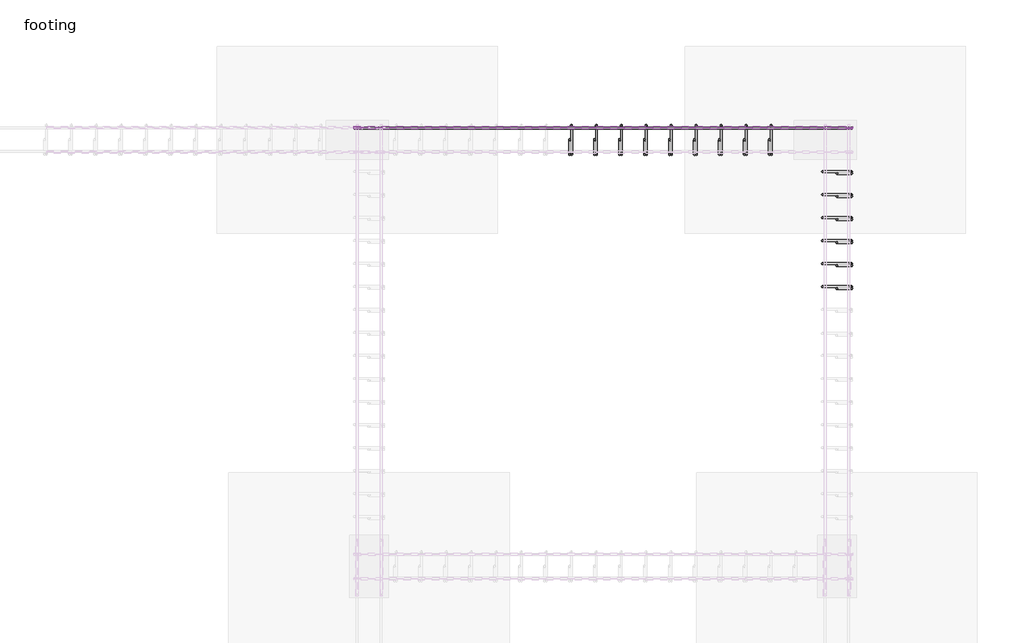
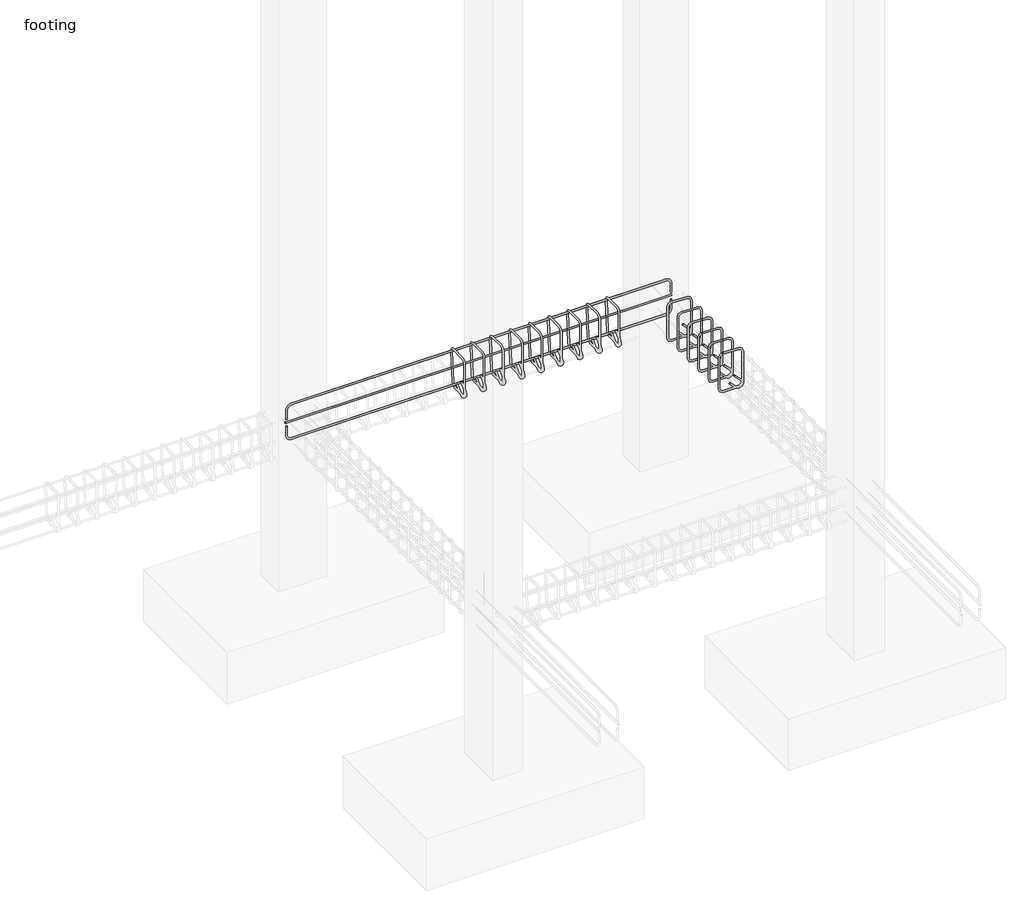
# One storey, part 21 of 21: 18 reinforcing bars.
"""IFC4 building model written with IfcOpenShell, lengths in millimetres."""

from ifc_helpers import new_model, si_unit, point, frame, origin, place, context, project, spatial, polyline, circle_curve, trimmed, segment, composite_curve, element, save
from ifc_brep_helpers import swept_disk

model = new_model("IFC4")

# Units and contexts
model_context = context("Model", 3, world=origin())
ifc_project = project(units=[si_unit("LENGTHUNIT", "METRE", prefix="MILLI")], contexts=[model_context])

# Site, building, storey
site = spatial("IfcSite", under=ifc_project)
building = spatial("IfcBuilding", under=site)
storey = spatial("IfcBuildingStorey", under=building, Name="footing", Elevation=-1524.0)

# Reinforcing bars
placement = place(None, origin())
element("IfcReinforcingBar", 1, at=placement, inside=storey, context=model_context, shape_type="SolidModel", body=[
    swept_disk(composite_curve([segment(polyline([(-4722.5521673, 11058.8872086, -236.1172592), (-4722.5521673, 11058.8872086, -312.3172592)]), True, "CONTINUOUS"), segment(trimmed(circle_curve(frame((-4767.0021673, 11058.8872086, -312.3172592), z_axis=(0.0, 1.0, -2.1166279873208456e-12), x_axis=(44.44999999999982, 0.0, 0.0)), 44.45), [point((-4722.5521673, 11058.8872086, -312.3172592))], [point((-4767.0021673, 11058.8872086, -356.7672592))], True, "CARTESIAN"), True, "CONTINUOUS"), segment(polyline([(-4767.0021673, 11058.8872086, -356.7672592), (-7917.3959173, 11058.8872086, -356.7672592)]), True, "CONTINUOUS"), segment(trimmed(circle_curve(frame((-7917.3959173, 11058.8872086, -312.3172592), z_axis=(0.0, 1.0, -2.1166279873208456e-12), x_axis=(0.0, 0.0, -44.44999999999999)), 44.45), [point((-7917.3959173, 11058.8872086, -356.7672592))], [point((-7961.8459173, 11058.8872086, -312.3172592))], True, "CARTESIAN"), True, "CONTINUOUS"), segment(polyline([(-7961.8459173, 11058.8872086, -312.3172592), (-7961.8459173, 11058.8872086, -236.1172592)]), True, "CONTINUOUS")], self_intersect=False), 6.35),
])
element("IfcReinforcingBar", 2, at=placement, inside=storey, context=model_context, shape_type="SolidModel", body=[
    swept_disk(composite_curve([segment(polyline([(-4722.5521673, 11058.8872086, -170.2827408), (-4722.5521673, 11058.8872086, -94.0827408)]), True, "CONTINUOUS"), segment(trimmed(circle_curve(frame((-4767.0021673, 11058.8872086, -94.0827408), z_axis=(0.0, -1.0, 0.0), x_axis=(44.44999999999982, 0.0, 0.0)), 44.45), [point((-4722.5521673, 11058.8872086, -94.0827408))], [point((-4767.0021673, 11058.8872086, -49.6327408))], True, "CARTESIAN"), True, "CONTINUOUS"), segment(polyline([(-4767.0021673, 11058.8872086, -49.6327408), (-7917.3959173, 11058.8872086, -49.6327408)]), True, "CONTINUOUS"), segment(trimmed(circle_curve(frame((-7917.3959173, 11058.8872086, -94.0827408), z_axis=(0.0, -1.0, 0.0), x_axis=(0.0, 0.0, 44.449999999999996)), 44.45), [point((-7917.3959173, 11058.8872086, -49.6327408))], [point((-7961.8459173, 11058.8872086, -94.0827408))], True, "CARTESIAN"), True, "CONTINUOUS"), segment(polyline([(-7961.8459173, 11058.8872086, -94.0827408), (-7961.8459173, 11058.8872086, -170.2827408)]), True, "CONTINUOUS")], self_intersect=False), 6.35),
])
element("IfcReinforcingBar", 3, at=placement, inside=storey, context=model_context, shape_type="SolidModel", body=[
    swept_disk(composite_curve([segment(polyline([(-4716.2021673, 11064.4668244, -203.2), (-7968.1959173, 11064.4668244, -203.2)]), True, "CONTINUOUS")], self_intersect=False), 6.35),
])
element("IfcReinforcingBar", 4, at=placement, inside=storey, context=model_context, shape_type="SolidModel", body=[
    swept_disk(composite_curve([segment(polyline([(-6560.8883428, 10994.9387132, -310.8825168), (-6560.8883428, 10940.0737147, -365.7475153)]), True, "CONTINUOUS"), segment(trimmed(circle_curve(frame((-6560.8883428, 10917.6230744, -343.296875), z_axis=(-1.0, 0.0, 0.0), x_axis=(0.0, 22.450640299999577, -22.450640299999975)), 31.75), [point((-6560.8883428, 10940.0737147, -365.7475153))], [point((-6560.8883428, 10885.8730744, -343.296875))], True, "CARTESIAN"), True, "CONTINUOUS"), segment(polyline([(-6560.8883428, 10885.8730744, -343.296875), (-6560.8883428, 10885.8730744, -63.103125)]), True, "CONTINUOUS"), segment(trimmed(circle_curve(frame((-6560.8883428, 10917.6230744, -63.103125), z_axis=(-1.0, 0.0, 0.0), x_axis=(0.0, -31.75, 0.0)), 31.75), [point((-6560.8883428, 10885.8730744, -63.103125))], [point((-6560.8883428, 10917.6230744, -31.353125))], True, "CARTESIAN"), True, "CONTINUOUS"), segment(polyline([(-6560.8883428, 10917.6230744, -31.353125), (-6560.8883428, 11045.4168244, -31.353125)]), True, "CONTINUOUS"), segment(trimmed(circle_curve(frame((-6559.7159328, 11045.4168244, -63.0814712), z_axis=(-0.9993179916193466, 0.0, -0.03692629992126919), x_axis=(-1.1724100000001272, 0.0, 31.728346200000004)), 31.75), [point((-6560.8883428, 11045.4168244, -31.353125))], [point((-6559.7159328, 11077.1668244, -63.0814712))], True, "CARTESIAN"), True, "CONTINUOUS"), segment(polyline([(-6559.7159328, 11077.1668244, -63.0814712), (-6549.3607528, 11077.1668244, -343.3185288)]), True, "CONTINUOUS"), segment(trimmed(circle_curve(frame((-6549.3607528, 11045.4168244, -343.3185288), z_axis=(-0.9993179916193466, 0.0, -0.03692629992126919), x_axis=(0.0, 31.75, 0.0)), 31.75), [point((-6549.3607528, 11077.1668244, -343.3185288))], [point((-6548.1883428, 11045.4168244, -375.046875))], True, "CARTESIAN"), True, "CONTINUOUS"), segment(polyline([(-6548.1883428, 11045.4168244, -375.046875), (-6548.1883428, 10917.6230744, -375.046875)]), True, "CONTINUOUS"), segment(trimmed(circle_curve(frame((-6548.1883428, 10917.6230744, -343.296875), z_axis=(-1.0, 0.0, 0.0), x_axis=(0.0, 0.0, -31.75)), 31.75), [point((-6548.1883428, 10917.6230744, -375.046875))], [point((-6548.1883428, 10895.1724341, -320.8462347))], True, "CARTESIAN"), True, "CONTINUOUS"), segment(polyline([(-6548.1883428, 10895.1724341, -320.8462347), (-6548.1883428, 10950.0374326, -265.9812362)]), True, "CONTINUOUS")], self_intersect=False), 6.35),
])
element("IfcReinforcingBar", 5, at=placement, inside=storey, context=model_context, shape_type="SolidModel", body=[
    swept_disk(composite_curve([segment(polyline([(-6398.1883428, 10994.9387132, -310.8825168), (-6398.1883428, 10940.0737147, -365.7475153)]), True, "CONTINUOUS"), segment(trimmed(circle_curve(frame((-6398.1883428, 10917.6230744, -343.296875), z_axis=(-1.0, 0.0, 0.0), x_axis=(0.0, 22.450640299999577, -22.450640299999975)), 31.75), [point((-6398.1883428, 10940.0737147, -365.7475153))], [point((-6398.1883428, 10885.8730744, -343.296875))], True, "CARTESIAN"), True, "CONTINUOUS"), segment(polyline([(-6398.1883428, 10885.8730744, -343.296875), (-6398.1883428, 10885.8730744, -63.103125)]), True, "CONTINUOUS"), segment(trimmed(circle_curve(frame((-6398.1883428, 10917.6230744, -63.103125), z_axis=(-1.0, 0.0, 0.0), x_axis=(0.0, -31.75, 0.0)), 31.75), [point((-6398.1883428, 10885.8730744, -63.103125))], [point((-6398.1883428, 10917.6230744, -31.353125))], True, "CARTESIAN"), True, "CONTINUOUS"), segment(polyline([(-6398.1883428, 10917.6230744, -31.353125), (-6398.1883428, 11045.4168244, -31.353125)]), True, "CONTINUOUS"), segment(trimmed(circle_curve(frame((-6397.0159328, 11045.4168244, -63.0814712), z_axis=(-0.9993179916193466, 0.0, -0.03692629992126919), x_axis=(-1.1724100000001272, 0.0, 31.728346200000004)), 31.75), [point((-6398.1883428, 11045.4168244, -31.353125))], [point((-6397.0159328, 11077.1668244, -63.0814712))], True, "CARTESIAN"), True, "CONTINUOUS"), segment(polyline([(-6397.0159328, 11077.1668244, -63.0814712), (-6386.6607528, 11077.1668244, -343.3185288)]), True, "CONTINUOUS"), segment(trimmed(circle_curve(frame((-6386.6607528, 11045.4168244, -343.3185288), z_axis=(-0.9993179916193466, 0.0, -0.03692629992126919), x_axis=(0.0, 31.75, 0.0)), 31.75), [point((-6386.6607528, 11077.1668244, -343.3185288))], [point((-6385.4883428, 11045.4168244, -375.046875))], True, "CARTESIAN"), True, "CONTINUOUS"), segment(polyline([(-6385.4883428, 11045.4168244, -375.046875), (-6385.4883428, 10917.6230744, -375.046875)]), True, "CONTINUOUS"), segment(trimmed(circle_curve(frame((-6385.4883428, 10917.6230744, -343.296875), z_axis=(-1.0, 0.0, 0.0), x_axis=(0.0, 0.0, -31.75)), 31.75), [point((-6385.4883428, 10917.6230744, -375.046875))], [point((-6385.4883428, 10895.1724341, -320.8462347))], True, "CARTESIAN"), True, "CONTINUOUS"), segment(polyline([(-6385.4883428, 10895.1724341, -320.8462347), (-6385.4883428, 10950.0374326, -265.9812362)]), True, "CONTINUOUS")], self_intersect=False), 6.35),
])
element("IfcReinforcingBar", 6, at=placement, inside=storey, context=model_context, shape_type="SolidModel", body=[
    swept_disk(composite_curve([segment(polyline([(-6235.4883428, 10994.9387132, -310.8825168), (-6235.4883428, 10940.0737147, -365.7475153)]), True, "CONTINUOUS"), segment(trimmed(circle_curve(frame((-6235.4883428, 10917.6230744, -343.296875), z_axis=(-1.0, 0.0, 0.0), x_axis=(0.0, 22.450640299999577, -22.450640299999975)), 31.75), [point((-6235.4883428, 10940.0737147, -365.7475153))], [point((-6235.4883428, 10885.8730744, -343.296875))], True, "CARTESIAN"), True, "CONTINUOUS"), segment(polyline([(-6235.4883428, 10885.8730744, -343.296875), (-6235.4883428, 10885.8730744, -63.103125)]), True, "CONTINUOUS"), segment(trimmed(circle_curve(frame((-6235.4883428, 10917.6230744, -63.103125), z_axis=(-1.0, 0.0, 0.0), x_axis=(0.0, -31.75, 0.0)), 31.75), [point((-6235.4883428, 10885.8730744, -63.103125))], [point((-6235.4883428, 10917.6230744, -31.353125))], True, "CARTESIAN"), True, "CONTINUOUS"), segment(polyline([(-6235.4883428, 10917.6230744, -31.353125), (-6235.4883428, 11045.4168244, -31.353125)]), True, "CONTINUOUS"), segment(trimmed(circle_curve(frame((-6234.3159328, 11045.4168244, -63.0814712), z_axis=(-0.9993179916193466, 0.0, -0.03692629992126919), x_axis=(-1.1724100000001272, 0.0, 31.728346200000004)), 31.75), [point((-6235.4883428, 11045.4168244, -31.353125))], [point((-6234.3159328, 11077.1668244, -63.0814712))], True, "CARTESIAN"), True, "CONTINUOUS"), segment(polyline([(-6234.3159328, 11077.1668244, -63.0814712), (-6223.9607528, 11077.1668244, -343.3185288)]), True, "CONTINUOUS"), segment(trimmed(circle_curve(frame((-6223.9607528, 11045.4168244, -343.3185288), z_axis=(-0.9993179916193466, 0.0, -0.03692629992126919), x_axis=(0.0, 31.75, 0.0)), 31.75), [point((-6223.9607528, 11077.1668244, -343.3185288))], [point((-6222.7883428, 11045.4168244, -375.046875))], True, "CARTESIAN"), True, "CONTINUOUS"), segment(polyline([(-6222.7883428, 11045.4168244, -375.046875), (-6222.7883428, 10917.6230744, -375.046875)]), True, "CONTINUOUS"), segment(trimmed(circle_curve(frame((-6222.7883428, 10917.6230744, -343.296875), z_axis=(-1.0, 0.0, 0.0), x_axis=(0.0, 0.0, -31.75)), 31.75), [point((-6222.7883428, 10917.6230744, -375.046875))], [point((-6222.7883428, 10895.1724341, -320.8462347))], True, "CARTESIAN"), True, "CONTINUOUS"), segment(polyline([(-6222.7883428, 10895.1724341, -320.8462347), (-6222.7883428, 10950.0374326, -265.9812362)]), True, "CONTINUOUS")], self_intersect=False), 6.35),
])
element("IfcReinforcingBar", 7, at=placement, inside=storey, context=model_context, shape_type="SolidModel", body=[
    swept_disk(composite_curve([segment(polyline([(-6072.7883428, 10994.9387132, -310.8825168), (-6072.7883428, 10940.0737147, -365.7475153)]), True, "CONTINUOUS"), segment(trimmed(circle_curve(frame((-6072.7883428, 10917.6230744, -343.296875), z_axis=(-1.0, 0.0, 0.0), x_axis=(0.0, 22.450640299999577, -22.450640299999975)), 31.75), [point((-6072.7883428, 10940.0737147, -365.7475153))], [point((-6072.7883428, 10885.8730744, -343.296875))], True, "CARTESIAN"), True, "CONTINUOUS"), segment(polyline([(-6072.7883428, 10885.8730744, -343.296875), (-6072.7883428, 10885.8730744, -63.103125)]), True, "CONTINUOUS"), segment(trimmed(circle_curve(frame((-6072.7883428, 10917.6230744, -63.103125), z_axis=(-1.0, 0.0, 0.0), x_axis=(0.0, -31.75, 0.0)), 31.75), [point((-6072.7883428, 10885.8730744, -63.103125))], [point((-6072.7883428, 10917.6230744, -31.353125))], True, "CARTESIAN"), True, "CONTINUOUS"), segment(polyline([(-6072.7883428, 10917.6230744, -31.353125), (-6072.7883428, 11045.4168244, -31.353125)]), True, "CONTINUOUS"), segment(trimmed(circle_curve(frame((-6071.6159328, 11045.4168244, -63.0814712), z_axis=(-0.9993179916193466, 0.0, -0.03692629992126919), x_axis=(-1.1724099999992177, 0.0, 31.728346200000004)), 31.75), [point((-6072.7883428, 11045.4168244, -31.353125))], [point((-6071.6159328, 11077.1668244, -63.0814712))], True, "CARTESIAN"), True, "CONTINUOUS"), segment(polyline([(-6071.6159328, 11077.1668244, -63.0814712), (-6061.2607528, 11077.1668244, -343.3185288)]), True, "CONTINUOUS"), segment(trimmed(circle_curve(frame((-6061.2607528, 11045.4168244, -343.3185288), z_axis=(-0.9993179916193466, 0.0, -0.03692629992126919), x_axis=(0.0, 31.75, 0.0)), 31.75), [point((-6061.2607528, 11077.1668244, -343.3185288))], [point((-6060.0883428, 11045.4168244, -375.046875))], True, "CARTESIAN"), True, "CONTINUOUS"), segment(polyline([(-6060.0883428, 11045.4168244, -375.046875), (-6060.0883428, 10917.6230744, -375.046875)]), True, "CONTINUOUS"), segment(trimmed(circle_curve(frame((-6060.0883428, 10917.6230744, -343.296875), z_axis=(-1.0, 0.0, 0.0), x_axis=(0.0, 0.0, -31.75)), 31.75), [point((-6060.0883428, 10917.6230744, -375.046875))], [point((-6060.0883428, 10895.1724341, -320.8462347))], True, "CARTESIAN"), True, "CONTINUOUS"), segment(polyline([(-6060.0883428, 10895.1724341, -320.8462347), (-6060.0883428, 10950.0374326, -265.9812362)]), True, "CONTINUOUS")], self_intersect=False), 6.35),
])
element("IfcReinforcingBar", 8, at=placement, inside=storey, context=model_context, shape_type="SolidModel", body=[
    swept_disk(composite_curve([segment(polyline([(-5910.0883428, 10994.9387132, -310.8825168), (-5910.0883428, 10940.0737147, -365.7475153)]), True, "CONTINUOUS"), segment(trimmed(circle_curve(frame((-5910.0883428, 10917.6230744, -343.296875), z_axis=(-1.0, 0.0, 0.0), x_axis=(0.0, 22.450640299999577, -22.450640299999975)), 31.75), [point((-5910.0883428, 10940.0737147, -365.7475153))], [point((-5910.0883428, 10885.8730744, -343.296875))], True, "CARTESIAN"), True, "CONTINUOUS"), segment(polyline([(-5910.0883428, 10885.8730744, -343.296875), (-5910.0883428, 10885.8730744, -63.103125)]), True, "CONTINUOUS"), segment(trimmed(circle_curve(frame((-5910.0883428, 10917.6230744, -63.103125), z_axis=(-1.0, 0.0, 0.0), x_axis=(0.0, -31.75, 0.0)), 31.75), [point((-5910.0883428, 10885.8730744, -63.103125))], [point((-5910.0883428, 10917.6230744, -31.353125))], True, "CARTESIAN"), True, "CONTINUOUS"), segment(polyline([(-5910.0883428, 10917.6230744, -31.353125), (-5910.0883428, 11045.4168244, -31.353125)]), True, "CONTINUOUS"), segment(trimmed(circle_curve(frame((-5908.9159328, 11045.4168244, -63.0814712), z_axis=(-0.9993179916193466, 0.0, -0.03692629992126919), x_axis=(-1.1724100000001272, 0.0, 31.728346200000004)), 31.75), [point((-5910.0883428, 11045.4168244, -31.353125))], [point((-5908.9159328, 11077.1668244, -63.0814712))], True, "CARTESIAN"), True, "CONTINUOUS"), segment(polyline([(-5908.9159328, 11077.1668244, -63.0814712), (-5898.5607528, 11077.1668244, -343.3185288)]), True, "CONTINUOUS"), segment(trimmed(circle_curve(frame((-5898.5607528, 11045.4168244, -343.3185288), z_axis=(-0.9993179916193466, 0.0, -0.03692629992126919), x_axis=(0.0, 31.75, 0.0)), 31.75), [point((-5898.5607528, 11077.1668244, -343.3185288))], [point((-5897.3883428, 11045.4168244, -375.046875))], True, "CARTESIAN"), True, "CONTINUOUS"), segment(polyline([(-5897.3883428, 11045.4168244, -375.046875), (-5897.3883428, 10917.6230744, -375.046875)]), True, "CONTINUOUS"), segment(trimmed(circle_curve(frame((-5897.3883428, 10917.6230744, -343.296875), z_axis=(-1.0, 0.0, 0.0), x_axis=(0.0, 0.0, -31.75)), 31.75), [point((-5897.3883428, 10917.6230744, -375.046875))], [point((-5897.3883428, 10895.1724341, -320.8462347))], True, "CARTESIAN"), True, "CONTINUOUS"), segment(polyline([(-5897.3883428, 10895.1724341, -320.8462347), (-5897.3883428, 10950.0374326, -265.9812362)]), True, "CONTINUOUS")], self_intersect=False), 6.35),
])
element("IfcReinforcingBar", 9, at=placement, inside=storey, context=model_context, shape_type="SolidModel", body=[
    swept_disk(composite_curve([segment(polyline([(-5747.3883428, 10994.9387132, -310.8825168), (-5747.3883428, 10940.0737147, -365.7475153)]), True, "CONTINUOUS"), segment(trimmed(circle_curve(frame((-5747.3883428, 10917.6230744, -343.296875), z_axis=(-1.0, 0.0, 0.0), x_axis=(0.0, 22.450640299999577, -22.450640299999975)), 31.75), [point((-5747.3883428, 10940.0737147, -365.7475153))], [point((-5747.3883428, 10885.8730744, -343.296875))], True, "CARTESIAN"), True, "CONTINUOUS"), segment(polyline([(-5747.3883428, 10885.8730744, -343.296875), (-5747.3883428, 10885.8730744, -63.103125)]), True, "CONTINUOUS"), segment(trimmed(circle_curve(frame((-5747.3883428, 10917.6230744, -63.103125), z_axis=(-1.0, 0.0, 0.0), x_axis=(0.0, -31.75, 0.0)), 31.75), [point((-5747.3883428, 10885.8730744, -63.103125))], [point((-5747.3883428, 10917.6230744, -31.353125))], True, "CARTESIAN"), True, "CONTINUOUS"), segment(polyline([(-5747.3883428, 10917.6230744, -31.353125), (-5747.3883428, 11045.4168244, -31.353125)]), True, "CONTINUOUS"), segment(trimmed(circle_curve(frame((-5746.2159328, 11045.4168244, -63.0814712), z_axis=(-0.9993179916193466, 0.0, -0.03692629992126919), x_axis=(-1.1724100000001272, 0.0, 31.728346200000004)), 31.75), [point((-5747.3883428, 11045.4168244, -31.353125))], [point((-5746.2159328, 11077.1668244, -63.0814712))], True, "CARTESIAN"), True, "CONTINUOUS"), segment(polyline([(-5746.2159328, 11077.1668244, -63.0814712), (-5735.8607528, 11077.1668244, -343.3185288)]), True, "CONTINUOUS"), segment(trimmed(circle_curve(frame((-5735.8607528, 11045.4168244, -343.3185288), z_axis=(-0.9993179916193466, 0.0, -0.03692629992126919), x_axis=(0.0, 31.75, 0.0)), 31.75), [point((-5735.8607528, 11077.1668244, -343.3185288))], [point((-5734.6883428, 11045.4168244, -375.046875))], True, "CARTESIAN"), True, "CONTINUOUS"), segment(polyline([(-5734.6883428, 11045.4168244, -375.046875), (-5734.6883428, 10917.6230744, -375.046875)]), True, "CONTINUOUS"), segment(trimmed(circle_curve(frame((-5734.6883428, 10917.6230744, -343.296875), z_axis=(-1.0, 0.0, 0.0), x_axis=(0.0, 0.0, -31.75)), 31.75), [point((-5734.6883428, 10917.6230744, -375.046875))], [point((-5734.6883428, 10895.1724341, -320.8462347))], True, "CARTESIAN"), True, "CONTINUOUS"), segment(polyline([(-5734.6883428, 10895.1724341, -320.8462347), (-5734.6883428, 10950.0374326, -265.9812362)]), True, "CONTINUOUS")], self_intersect=False), 6.35),
])
element("IfcReinforcingBar", 10, at=placement, inside=storey, context=model_context, shape_type="SolidModel", body=[
    swept_disk(composite_curve([segment(polyline([(-5584.6883428, 10994.9387132, -310.8825168), (-5584.6883428, 10940.0737147, -365.7475153)]), True, "CONTINUOUS"), segment(trimmed(circle_curve(frame((-5584.6883428, 10917.6230744, -343.296875), z_axis=(-1.0, 0.0, 0.0), x_axis=(0.0, 22.450640299999577, -22.450640299999975)), 31.75), [point((-5584.6883428, 10940.0737147, -365.7475153))], [point((-5584.6883428, 10885.8730744, -343.296875))], True, "CARTESIAN"), True, "CONTINUOUS"), segment(polyline([(-5584.6883428, 10885.8730744, -343.296875), (-5584.6883428, 10885.8730744, -63.103125)]), True, "CONTINUOUS"), segment(trimmed(circle_curve(frame((-5584.6883428, 10917.6230744, -63.103125), z_axis=(-1.0, 0.0, 0.0), x_axis=(0.0, -31.75, 0.0)), 31.75), [point((-5584.6883428, 10885.8730744, -63.103125))], [point((-5584.6883428, 10917.6230744, -31.353125))], True, "CARTESIAN"), True, "CONTINUOUS"), segment(polyline([(-5584.6883428, 10917.6230744, -31.353125), (-5584.6883428, 11045.4168244, -31.353125)]), True, "CONTINUOUS"), segment(trimmed(circle_curve(frame((-5583.5159328, 11045.4168244, -63.0814712), z_axis=(-0.9993179916193466, 0.0, -0.03692629992126919), x_axis=(-1.1724100000001272, 0.0, 31.728346200000004)), 31.75), [point((-5584.6883428, 11045.4168244, -31.353125))], [point((-5583.5159328, 11077.1668244, -63.0814712))], True, "CARTESIAN"), True, "CONTINUOUS"), segment(polyline([(-5583.5159328, 11077.1668244, -63.0814712), (-5573.1607528, 11077.1668244, -343.3185288)]), True, "CONTINUOUS"), segment(trimmed(circle_curve(frame((-5573.1607528, 11045.4168244, -343.3185288), z_axis=(-0.9993179916193466, 0.0, -0.03692629992126919), x_axis=(0.0, 31.75, 0.0)), 31.75), [point((-5573.1607528, 11077.1668244, -343.3185288))], [point((-5571.9883428, 11045.4168244, -375.046875))], True, "CARTESIAN"), True, "CONTINUOUS"), segment(polyline([(-5571.9883428, 11045.4168244, -375.046875), (-5571.9883428, 10917.6230744, -375.046875)]), True, "CONTINUOUS"), segment(trimmed(circle_curve(frame((-5571.9883428, 10917.6230744, -343.296875), z_axis=(-1.0, 0.0, 0.0), x_axis=(0.0, 0.0, -31.75)), 31.75), [point((-5571.9883428, 10917.6230744, -375.046875))], [point((-5571.9883428, 10895.1724341, -320.8462347))], True, "CARTESIAN"), True, "CONTINUOUS"), segment(polyline([(-5571.9883428, 10895.1724341, -320.8462347), (-5571.9883428, 10950.0374326, -265.9812362)]), True, "CONTINUOUS")], self_intersect=False), 6.35),
])
element("IfcReinforcingBar", 11, at=placement, inside=storey, context=model_context, shape_type="SolidModel", body=[
    swept_disk(composite_curve([segment(polyline([(-5421.9883428, 10994.9387132, -310.8825168), (-5421.9883428, 10940.0737147, -365.7475153)]), True, "CONTINUOUS"), segment(trimmed(circle_curve(frame((-5421.9883428, 10917.6230744, -343.296875), z_axis=(-1.0, 0.0, 0.0), x_axis=(0.0, 22.450640299999577, -22.450640299999975)), 31.75), [point((-5421.9883428, 10940.0737147, -365.7475153))], [point((-5421.9883428, 10885.8730744, -343.296875))], True, "CARTESIAN"), True, "CONTINUOUS"), segment(polyline([(-5421.9883428, 10885.8730744, -343.296875), (-5421.9883428, 10885.8730744, -63.103125)]), True, "CONTINUOUS"), segment(trimmed(circle_curve(frame((-5421.9883428, 10917.6230744, -63.103125), z_axis=(-1.0, 0.0, 0.0), x_axis=(0.0, -31.75, 0.0)), 31.75), [point((-5421.9883428, 10885.8730744, -63.103125))], [point((-5421.9883428, 10917.6230744, -31.353125))], True, "CARTESIAN"), True, "CONTINUOUS"), segment(polyline([(-5421.9883428, 10917.6230744, -31.353125), (-5421.9883428, 11045.4168244, -31.353125)]), True, "CONTINUOUS"), segment(trimmed(circle_curve(frame((-5420.8159328, 11045.4168244, -63.0814712), z_axis=(-0.9993179916193466, 0.0, -0.03692629992126919), x_axis=(-1.1724100000001272, 0.0, 31.728346200000004)), 31.75), [point((-5421.9883428, 11045.4168244, -31.353125))], [point((-5420.8159328, 11077.1668244, -63.0814712))], True, "CARTESIAN"), True, "CONTINUOUS"), segment(polyline([(-5420.8159328, 11077.1668244, -63.0814712), (-5410.4607528, 11077.1668244, -343.3185288)]), True, "CONTINUOUS"), segment(trimmed(circle_curve(frame((-5410.4607528, 11045.4168244, -343.3185288), z_axis=(-0.9993179916193466, 0.0, -0.03692629992126919), x_axis=(0.0, 31.75, 0.0)), 31.75), [point((-5410.4607528, 11077.1668244, -343.3185288))], [point((-5409.2883428, 11045.4168244, -375.046875))], True, "CARTESIAN"), True, "CONTINUOUS"), segment(polyline([(-5409.2883428, 11045.4168244, -375.046875), (-5409.2883428, 10917.6230744, -375.046875)]), True, "CONTINUOUS"), segment(trimmed(circle_curve(frame((-5409.2883428, 10917.6230744, -343.296875), z_axis=(-1.0, 0.0, 0.0), x_axis=(0.0, 0.0, -31.75)), 31.75), [point((-5409.2883428, 10917.6230744, -375.046875))], [point((-5409.2883428, 10895.1724341, -320.8462347))], True, "CARTESIAN"), True, "CONTINUOUS"), segment(polyline([(-5409.2883428, 10895.1724341, -320.8462347), (-5409.2883428, 10950.0374326, -265.9812362)]), True, "CONTINUOUS")], self_intersect=False), 6.35),
])
element("IfcReinforcingBar", 12, at=placement, inside=storey, context=model_context, shape_type="SolidModel", body=[
    swept_disk(composite_curve([segment(polyline([(-5259.2883428, 10994.9387132, -310.8825168), (-5259.2883428, 10940.0737147, -365.7475153)]), True, "CONTINUOUS"), segment(trimmed(circle_curve(frame((-5259.2883428, 10917.6230744, -343.296875), z_axis=(-1.0, 0.0, 0.0), x_axis=(0.0, 22.450640299999577, -22.450640299999975)), 31.75), [point((-5259.2883428, 10940.0737147, -365.7475153))], [point((-5259.2883428, 10885.8730744, -343.296875))], True, "CARTESIAN"), True, "CONTINUOUS"), segment(polyline([(-5259.2883428, 10885.8730744, -343.296875), (-5259.2883428, 10885.8730744, -63.103125)]), True, "CONTINUOUS"), segment(trimmed(circle_curve(frame((-5259.2883428, 10917.6230744, -63.103125), z_axis=(-1.0, 0.0, 0.0), x_axis=(0.0, -31.75, 0.0)), 31.75), [point((-5259.2883428, 10885.8730744, -63.103125))], [point((-5259.2883428, 10917.6230744, -31.353125))], True, "CARTESIAN"), True, "CONTINUOUS"), segment(polyline([(-5259.2883428, 10917.6230744, -31.353125), (-5259.2883428, 11045.4168244, -31.353125)]), True, "CONTINUOUS"), segment(trimmed(circle_curve(frame((-5258.1159328, 11045.4168244, -63.0814712), z_axis=(-0.9993179916193466, 0.0, -0.03692629992126919), x_axis=(-1.1724099999992177, 0.0, 31.728346200000004)), 31.75), [point((-5259.2883428, 11045.4168244, -31.353125))], [point((-5258.1159328, 11077.1668244, -63.0814712))], True, "CARTESIAN"), True, "CONTINUOUS"), segment(polyline([(-5258.1159328, 11077.1668244, -63.0814712), (-5247.7607528, 11077.1668244, -343.3185288)]), True, "CONTINUOUS"), segment(trimmed(circle_curve(frame((-5247.7607528, 11045.4168244, -343.3185288), z_axis=(-0.9993179916193466, 0.0, -0.03692629992126919), x_axis=(0.0, 31.75, 0.0)), 31.75), [point((-5247.7607528, 11077.1668244, -343.3185288))], [point((-5246.5883428, 11045.4168244, -375.046875))], True, "CARTESIAN"), True, "CONTINUOUS"), segment(polyline([(-5246.5883428, 11045.4168244, -375.046875), (-5246.5883428, 10917.6230744, -375.046875)]), True, "CONTINUOUS"), segment(trimmed(circle_curve(frame((-5246.5883428, 10917.6230744, -343.296875), z_axis=(-1.0, 0.0, 0.0), x_axis=(0.0, 0.0, -31.75)), 31.75), [point((-5246.5883428, 10917.6230744, -375.046875))], [point((-5246.5883428, 10895.1724341, -320.8462347))], True, "CARTESIAN"), True, "CONTINUOUS"), segment(polyline([(-5246.5883428, 10895.1724341, -320.8462347), (-5246.5883428, 10950.0374326, -265.9812362)]), True, "CONTINUOUS")], self_intersect=False), 6.35),
])
element("IfcReinforcingBar", 13, at=placement, inside=storey, context=model_context, shape_type="SolidModel", body=[
    swept_disk(composite_curve([segment(polyline([(-4786.7165254, 10025.2699494, -265.9812362), (-4731.851527, 10025.2699494, -320.8462347)]), True, "CONTINUOUS"), segment(trimmed(circle_curve(frame((-4754.3021673, 10025.2699494, -343.296875), z_axis=(0.0, 1.0, 0.0), x_axis=(22.450640300000487, 0.0, 22.450640299999975)), 31.75), [point((-4731.851527, 10025.2699494, -320.8462347))], [point((-4754.3021673, 10025.2699494, -375.046875))], True, "CARTESIAN"), True, "CONTINUOUS"), segment(polyline([(-4754.3021673, 10025.2699494, -375.046875), (-4882.0959173, 10025.2699494, -375.046875)]), True, "CONTINUOUS"), segment(trimmed(circle_curve(frame((-4882.0959173, 10025.2699494, -343.296875), z_axis=(0.0, 1.0, 0.0), x_axis=(0.0, 0.0, -31.75)), 31.75), [point((-4882.0959173, 10025.2699494, -375.046875))], [point((-4913.8459173, 10025.2699494, -343.296875))], True, "CARTESIAN"), True, "CONTINUOUS"), segment(polyline([(-4913.8459173, 10025.2699494, -343.296875), (-4913.8459173, 10025.2699494, -63.103125)]), True, "CONTINUOUS"), segment(trimmed(circle_curve(frame((-4882.165658, 10023.1666957, -63.103125), z_axis=(0.06624421176864137, 0.9978034397651431, 0.0), x_axis=(-31.680259300000216, 2.103253700001005, 0.0)), 31.75), [point((-4913.8459173, 10025.2699494, -63.103125))], [point((-4882.165658, 10023.1666957, -31.353125))], True, "CARTESIAN"), True, "CONTINUOUS"), segment(polyline([(-4882.165658, 10023.1666957, -31.353125), (-4754.2324265, 10014.6732031, -31.353125)]), True, "CONTINUOUS"), segment(trimmed(circle_curve(frame((-4754.2324265, 10014.6732031, -63.103125), z_axis=(0.06624421176864137, 0.9978034397651431, 0.0), x_axis=(0.0, 0.0, 31.75)), 31.75), [point((-4754.2324265, 10014.6732031, -31.353125))], [point((-4722.5521673, 10012.5699494, -63.103125))], True, "CARTESIAN"), True, "CONTINUOUS"), segment(polyline([(-4722.5521673, 10012.5699494, -63.103125), (-4722.5521673, 10012.5699494, -343.296875)]), True, "CONTINUOUS"), segment(trimmed(circle_curve(frame((-4754.3021673, 10012.5699494, -343.296875), z_axis=(0.0, 1.0, 0.0), x_axis=(31.75, 0.0, 0.0)), 31.75), [point((-4722.5521673, 10012.5699494, -343.296875))], [point((-4776.7528076, 10012.5699494, -365.7475153))], True, "CARTESIAN"), True, "CONTINUOUS"), segment(polyline([(-4776.7528076, 10012.5699494, -365.7475153), (-4831.617806, 10012.5699494, -310.8825168)]), True, "CONTINUOUS")], self_intersect=False), 6.35),
])
element("IfcReinforcingBar", 14, at=placement, inside=storey, context=model_context, shape_type="SolidModel", body=[
    swept_disk(composite_curve([segment(polyline([(-4786.7165254, 10175.2699494, -265.9812362), (-4731.851527, 10175.2699494, -320.8462347)]), True, "CONTINUOUS"), segment(trimmed(circle_curve(frame((-4754.3021673, 10175.2699494, -343.296875), z_axis=(0.0, 1.0, 0.0), x_axis=(22.450640300000487, 0.0, 22.450640299999975)), 31.75), [point((-4731.851527, 10175.2699494, -320.8462347))], [point((-4754.3021673, 10175.2699494, -375.046875))], True, "CARTESIAN"), True, "CONTINUOUS"), segment(polyline([(-4754.3021673, 10175.2699494, -375.046875), (-4882.0959173, 10175.2699494, -375.046875)]), True, "CONTINUOUS"), segment(trimmed(circle_curve(frame((-4882.0959173, 10175.2699494, -343.296875), z_axis=(0.0, 1.0, 0.0), x_axis=(0.0, 0.0, -31.75)), 31.75), [point((-4882.0959173, 10175.2699494, -375.046875))], [point((-4913.8459173, 10175.2699494, -343.296875))], True, "CARTESIAN"), True, "CONTINUOUS"), segment(polyline([(-4913.8459173, 10175.2699494, -343.296875), (-4913.8459173, 10175.2699494, -63.103125)]), True, "CONTINUOUS"), segment(trimmed(circle_curve(frame((-4882.165658, 10173.1666957, -63.103125), z_axis=(0.06624421176864137, 0.9978034397651431, 0.0), x_axis=(-31.680259300000216, 2.103253700001005, 0.0)), 31.75), [point((-4913.8459173, 10175.2699494, -63.103125))], [point((-4882.165658, 10173.1666957, -31.353125))], True, "CARTESIAN"), True, "CONTINUOUS"), segment(polyline([(-4882.165658, 10173.1666957, -31.353125), (-4754.2324265, 10164.6732031, -31.353125)]), True, "CONTINUOUS"), segment(trimmed(circle_curve(frame((-4754.2324265, 10164.6732031, -63.103125), z_axis=(0.06624421176864137, 0.9978034397651431, 0.0), x_axis=(0.0, 0.0, 31.75)), 31.75), [point((-4754.2324265, 10164.6732031, -31.353125))], [point((-4722.5521673, 10162.5699494, -63.103125))], True, "CARTESIAN"), True, "CONTINUOUS"), segment(polyline([(-4722.5521673, 10162.5699494, -63.103125), (-4722.5521673, 10162.5699494, -343.296875)]), True, "CONTINUOUS"), segment(trimmed(circle_curve(frame((-4754.3021673, 10162.5699494, -343.296875), z_axis=(0.0, 1.0, 0.0), x_axis=(31.75, 0.0, 0.0)), 31.75), [point((-4722.5521673, 10162.5699494, -343.296875))], [point((-4776.7528076, 10162.5699494, -365.7475153))], True, "CARTESIAN"), True, "CONTINUOUS"), segment(polyline([(-4776.7528076, 10162.5699494, -365.7475153), (-4831.617806, 10162.5699494, -310.8825168)]), True, "CONTINUOUS")], self_intersect=False), 6.35),
])
element("IfcReinforcingBar", 15, at=placement, inside=storey, context=model_context, shape_type="SolidModel", body=[
    swept_disk(composite_curve([segment(polyline([(-4786.7165254, 10325.2699494, -265.9812362), (-4731.851527, 10325.2699494, -320.8462347)]), True, "CONTINUOUS"), segment(trimmed(circle_curve(frame((-4754.3021673, 10325.2699494, -343.296875), z_axis=(0.0, 1.0, 0.0), x_axis=(22.450640300000487, 0.0, 22.450640299999975)), 31.75), [point((-4731.851527, 10325.2699494, -320.8462347))], [point((-4754.3021673, 10325.2699494, -375.046875))], True, "CARTESIAN"), True, "CONTINUOUS"), segment(polyline([(-4754.3021673, 10325.2699494, -375.046875), (-4882.0959173, 10325.2699494, -375.046875)]), True, "CONTINUOUS"), segment(trimmed(circle_curve(frame((-4882.0959173, 10325.2699494, -343.296875), z_axis=(0.0, 1.0, 0.0), x_axis=(0.0, 0.0, -31.75)), 31.75), [point((-4882.0959173, 10325.2699494, -375.046875))], [point((-4913.8459173, 10325.2699494, -343.296875))], True, "CARTESIAN"), True, "CONTINUOUS"), segment(polyline([(-4913.8459173, 10325.2699494, -343.296875), (-4913.8459173, 10325.2699494, -63.103125)]), True, "CONTINUOUS"), segment(trimmed(circle_curve(frame((-4882.165658, 10323.1666957, -63.103125), z_axis=(0.06624421176864137, 0.9978034397651431, 0.0), x_axis=(-31.680259300000216, 2.103253700001005, 0.0)), 31.75), [point((-4913.8459173, 10325.2699494, -63.103125))], [point((-4882.165658, 10323.1666957, -31.353125))], True, "CARTESIAN"), True, "CONTINUOUS"), segment(polyline([(-4882.165658, 10323.1666957, -31.353125), (-4754.2324265, 10314.6732031, -31.353125)]), True, "CONTINUOUS"), segment(trimmed(circle_curve(frame((-4754.2324265, 10314.6732031, -63.103125), z_axis=(0.06624421176864137, 0.9978034397651431, 0.0), x_axis=(0.0, 0.0, 31.75)), 31.75), [point((-4754.2324265, 10314.6732031, -31.353125))], [point((-4722.5521673, 10312.5699494, -63.103125))], True, "CARTESIAN"), True, "CONTINUOUS"), segment(polyline([(-4722.5521673, 10312.5699494, -63.103125), (-4722.5521673, 10312.5699494, -343.296875)]), True, "CONTINUOUS"), segment(trimmed(circle_curve(frame((-4754.3021673, 10312.5699494, -343.296875), z_axis=(0.0, 1.0, 0.0), x_axis=(31.75, 0.0, 0.0)), 31.75), [point((-4722.5521673, 10312.5699494, -343.296875))], [point((-4776.7528076, 10312.5699494, -365.7475153))], True, "CARTESIAN"), True, "CONTINUOUS"), segment(polyline([(-4776.7528076, 10312.5699494, -365.7475153), (-4831.617806, 10312.5699494, -310.8825168)]), True, "CONTINUOUS")], self_intersect=False), 6.35),
])
element("IfcReinforcingBar", 16, at=placement, inside=storey, context=model_context, shape_type="SolidModel", body=[
    swept_disk(composite_curve([segment(polyline([(-4786.7165254, 10475.2699494, -265.9812362), (-4731.851527, 10475.2699494, -320.8462347)]), True, "CONTINUOUS"), segment(trimmed(circle_curve(frame((-4754.3021673, 10475.2699494, -343.296875), z_axis=(0.0, 1.0, 0.0), x_axis=(22.450640300000487, 0.0, 22.450640299999975)), 31.75), [point((-4731.851527, 10475.2699494, -320.8462347))], [point((-4754.3021673, 10475.2699494, -375.046875))], True, "CARTESIAN"), True, "CONTINUOUS"), segment(polyline([(-4754.3021673, 10475.2699494, -375.046875), (-4882.0959173, 10475.2699494, -375.046875)]), True, "CONTINUOUS"), segment(trimmed(circle_curve(frame((-4882.0959173, 10475.2699494, -343.296875), z_axis=(0.0, 1.0, 0.0), x_axis=(0.0, 0.0, -31.75)), 31.75), [point((-4882.0959173, 10475.2699494, -375.046875))], [point((-4913.8459173, 10475.2699494, -343.296875))], True, "CARTESIAN"), True, "CONTINUOUS"), segment(polyline([(-4913.8459173, 10475.2699494, -343.296875), (-4913.8459173, 10475.2699494, -63.103125)]), True, "CONTINUOUS"), segment(trimmed(circle_curve(frame((-4882.165658, 10473.1666957, -63.103125), z_axis=(0.06624421176864137, 0.9978034397651431, 0.0), x_axis=(-31.680259300000216, 2.103253700001005, 0.0)), 31.75), [point((-4913.8459173, 10475.2699494, -63.103125))], [point((-4882.165658, 10473.1666957, -31.353125))], True, "CARTESIAN"), True, "CONTINUOUS"), segment(polyline([(-4882.165658, 10473.1666957, -31.353125), (-4754.2324265, 10464.6732031, -31.353125)]), True, "CONTINUOUS"), segment(trimmed(circle_curve(frame((-4754.2324265, 10464.6732031, -63.103125), z_axis=(0.06624421176864137, 0.9978034397651431, 0.0), x_axis=(0.0, 0.0, 31.75)), 31.75), [point((-4754.2324265, 10464.6732031, -31.353125))], [point((-4722.5521673, 10462.5699494, -63.103125))], True, "CARTESIAN"), True, "CONTINUOUS"), segment(polyline([(-4722.5521673, 10462.5699494, -63.103125), (-4722.5521673, 10462.5699494, -343.296875)]), True, "CONTINUOUS"), segment(trimmed(circle_curve(frame((-4754.3021673, 10462.5699494, -343.296875), z_axis=(0.0, 1.0, 0.0), x_axis=(31.75, 0.0, 0.0)), 31.75), [point((-4722.5521673, 10462.5699494, -343.296875))], [point((-4776.7528076, 10462.5699494, -365.7475153))], True, "CARTESIAN"), True, "CONTINUOUS"), segment(polyline([(-4776.7528076, 10462.5699494, -365.7475153), (-4831.617806, 10462.5699494, -310.8825168)]), True, "CONTINUOUS")], self_intersect=False), 6.35),
])
element("IfcReinforcingBar", 17, at=placement, inside=storey, context=model_context, shape_type="SolidModel", body=[
    swept_disk(composite_curve([segment(polyline([(-4786.7165254, 10625.2699494, -265.9812362), (-4731.851527, 10625.2699494, -320.8462347)]), True, "CONTINUOUS"), segment(trimmed(circle_curve(frame((-4754.3021673, 10625.2699494, -343.296875), z_axis=(0.0, 1.0, 0.0), x_axis=(22.450640300000487, 0.0, 22.450640299999975)), 31.75), [point((-4731.851527, 10625.2699494, -320.8462347))], [point((-4754.3021673, 10625.2699494, -375.046875))], True, "CARTESIAN"), True, "CONTINUOUS"), segment(polyline([(-4754.3021673, 10625.2699494, -375.046875), (-4882.0959173, 10625.2699494, -375.046875)]), True, "CONTINUOUS"), segment(trimmed(circle_curve(frame((-4882.0959173, 10625.2699494, -343.296875), z_axis=(0.0, 1.0, 0.0), x_axis=(0.0, 0.0, -31.75)), 31.75), [point((-4882.0959173, 10625.2699494, -375.046875))], [point((-4913.8459173, 10625.2699494, -343.296875))], True, "CARTESIAN"), True, "CONTINUOUS"), segment(polyline([(-4913.8459173, 10625.2699494, -343.296875), (-4913.8459173, 10625.2699494, -63.103125)]), True, "CONTINUOUS"), segment(trimmed(circle_curve(frame((-4882.165658, 10623.1666957, -63.103125), z_axis=(0.06624421176864137, 0.9978034397651431, 0.0), x_axis=(-31.680259300000216, 2.103253700001005, 0.0)), 31.75), [point((-4913.8459173, 10625.2699494, -63.103125))], [point((-4882.165658, 10623.1666957, -31.353125))], True, "CARTESIAN"), True, "CONTINUOUS"), segment(polyline([(-4882.165658, 10623.1666957, -31.353125), (-4754.2324265, 10614.6732031, -31.353125)]), True, "CONTINUOUS"), segment(trimmed(circle_curve(frame((-4754.2324265, 10614.6732031, -63.103125), z_axis=(0.06624421176864137, 0.9978034397651431, 0.0), x_axis=(0.0, 0.0, 31.75)), 31.75), [point((-4754.2324265, 10614.6732031, -31.353125))], [point((-4722.5521673, 10612.5699494, -63.103125))], True, "CARTESIAN"), True, "CONTINUOUS"), segment(polyline([(-4722.5521673, 10612.5699494, -63.103125), (-4722.5521673, 10612.5699494, -343.296875)]), True, "CONTINUOUS"), segment(trimmed(circle_curve(frame((-4754.3021673, 10612.5699494, -343.296875), z_axis=(0.0, 1.0, 0.0), x_axis=(31.75, 0.0, 0.0)), 31.75), [point((-4722.5521673, 10612.5699494, -343.296875))], [point((-4776.7528076, 10612.5699494, -365.7475153))], True, "CARTESIAN"), True, "CONTINUOUS"), segment(polyline([(-4776.7528076, 10612.5699494, -365.7475153), (-4831.617806, 10612.5699494, -310.8825168)]), True, "CONTINUOUS")], self_intersect=False), 6.35),
])
element("IfcReinforcingBar", 18, at=placement, inside=storey, context=model_context, shape_type="SolidModel", body=[
    swept_disk(composite_curve([segment(polyline([(-4786.7165254, 10775.2699494, -265.9812362), (-4731.851527, 10775.2699494, -320.8462347)]), True, "CONTINUOUS"), segment(trimmed(circle_curve(frame((-4754.3021673, 10775.2699494, -343.296875), z_axis=(0.0, 1.0, 0.0), x_axis=(22.450640300000487, 0.0, 22.450640299999975)), 31.75), [point((-4731.851527, 10775.2699494, -320.8462347))], [point((-4754.3021673, 10775.2699494, -375.046875))], True, "CARTESIAN"), True, "CONTINUOUS"), segment(polyline([(-4754.3021673, 10775.2699494, -375.046875), (-4882.0959173, 10775.2699494, -375.046875)]), True, "CONTINUOUS"), segment(trimmed(circle_curve(frame((-4882.0959173, 10775.2699494, -343.296875), z_axis=(0.0, 1.0, 0.0), x_axis=(0.0, 0.0, -31.75)), 31.75), [point((-4882.0959173, 10775.2699494, -375.046875))], [point((-4913.8459173, 10775.2699494, -343.296875))], True, "CARTESIAN"), True, "CONTINUOUS"), segment(polyline([(-4913.8459173, 10775.2699494, -343.296875), (-4913.8459173, 10775.2699494, -63.103125)]), True, "CONTINUOUS"), segment(trimmed(circle_curve(frame((-4882.165658, 10773.1666957, -63.103125), z_axis=(0.06624421176864137, 0.9978034397651431, 0.0), x_axis=(-31.680259300000216, 2.103253700001005, 0.0)), 31.75), [point((-4913.8459173, 10775.2699494, -63.103125))], [point((-4882.165658, 10773.1666957, -31.353125))], True, "CARTESIAN"), True, "CONTINUOUS"), segment(polyline([(-4882.165658, 10773.1666957, -31.353125), (-4754.2324265, 10764.6732031, -31.353125)]), True, "CONTINUOUS"), segment(trimmed(circle_curve(frame((-4754.2324265, 10764.6732031, -63.103125), z_axis=(0.06624421176864137, 0.9978034397651431, 0.0), x_axis=(0.0, 0.0, 31.75)), 31.75), [point((-4754.2324265, 10764.6732031, -31.353125))], [point((-4722.5521673, 10762.5699494, -63.103125))], True, "CARTESIAN"), True, "CONTINUOUS"), segment(polyline([(-4722.5521673, 10762.5699494, -63.103125), (-4722.5521673, 10762.5699494, -343.296875)]), True, "CONTINUOUS"), segment(trimmed(circle_curve(frame((-4754.3021673, 10762.5699494, -343.296875), z_axis=(0.0, 1.0, 0.0), x_axis=(31.75, 0.0, 0.0)), 31.75), [point((-4722.5521673, 10762.5699494, -343.296875))], [point((-4776.7528076, 10762.5699494, -365.7475153))], True, "CARTESIAN"), True, "CONTINUOUS"), segment(polyline([(-4776.7528076, 10762.5699494, -365.7475153), (-4831.617806, 10762.5699494, -310.8825168)]), True, "CONTINUOUS")], self_intersect=False), 6.35),
])

save(model, "model.ifc")

# Revit data of these elements
# Elements 1, 2, 3, 4, 5, 6, 7, 8, 9, 10, 11, 12, 13, 14, 15, 16, 17, 18 (IfcReinforcingBar)
#   Phase Created = New Construction
